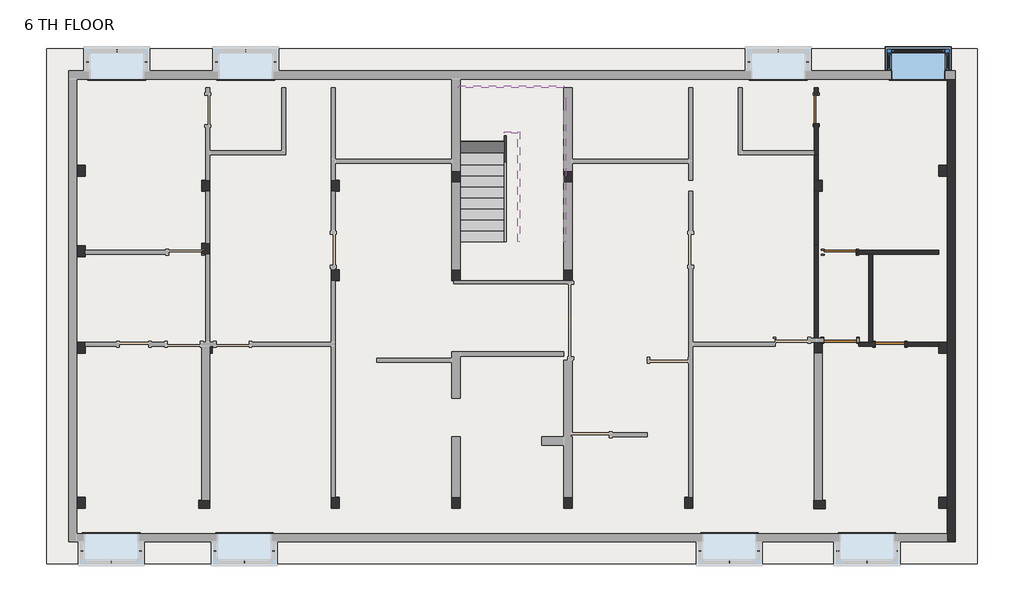
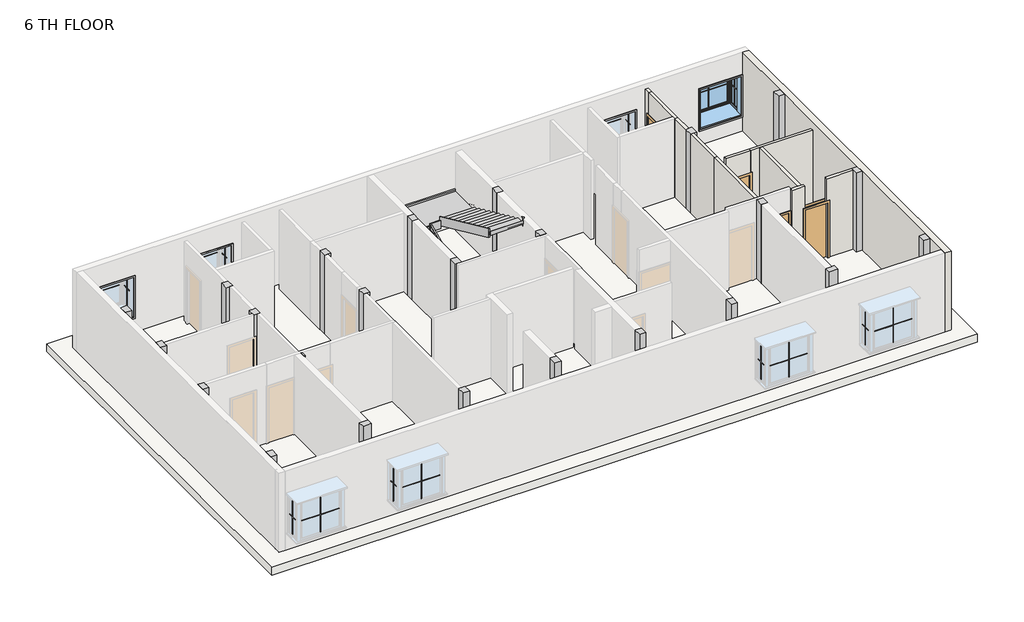
# One storey, part 2 of 2: 32 proxies, 24 columns, 11 walls, 6 members, 4 doors, 1 slab, 1 stair flight, 1 window.
"""IFC4 building model written with IfcOpenShell, lengths in millimetres."""

from ifc_helpers import new_model, si_unit, frame, origin, place, context, project, spatial, polyline, outline, extrude, faceted_brep, transform, mapped, element, save
from components import m_muntin_pattern_2x2_m_muntin_pattern_2x2_c1fd4460, m_muntin_pattern_2x2_m_muntin_pattern_2x2_777b163a, m_trim_window_interior_flat_picture_frame_44e8afef, column_1c121444, door_1991e9a2, door_a431d384, door_82def9da, m_door_single_panel_3_x7_f8176753, stair_flight_f18b4829, window_19bbd869

model = new_model("IFC4")

# Units and contexts
model_context = context("Model", 3, world=origin())
ifc_project = project(units=[si_unit("LENGTHUNIT", "METRE", prefix="MILLI")], contexts=[model_context])

# Site, building, storey
site = spatial("IfcSite", under=ifc_project)
building = spatial("IfcBuilding", under=site)
storey = spatial("IfcBuildingStorey", under=building, Name="6 TH FLOOR", Elevation=22402.8)

# Proxies
placement = place(None, origin())
m_muntin_pattern_2x2_m_muntin_pattern_2x2_shape = m_muntin_pattern_2x2_m_muntin_pattern_2x2_c1fd4460(model_context)
element("IfcBuildingElementProxy", 1, Name="M_Muntin Pattern_2x2 : M_Muntin Pattern_2x2", ObjectType="M_Muntin Pattern_2x2 : M_Muntin Pattern_2x2", at=placement, inside=storey, context=model_context, shape_type="MappedRepresentation", body=[
    mapped(m_muntin_pattern_2x2_m_muntin_pattern_2x2_shape, transform((-11500.7987957, -5499.9182661, 23123.45), x_axis=(-1.0, 0.0, 0.0), y_axis=(0.0, -1.0, 0.0), z_axis=(0.0, 0.0, 1.0))),
])
element("IfcBuildingElementProxy", 2, Name="M_Muntin Pattern_2x2 : M_Muntin Pattern_2x2", ObjectType="M_Muntin Pattern_2x2 : M_Muntin Pattern_2x2", at=placement, inside=storey, context=model_context, shape_type="MappedRepresentation", body=[
    mapped(m_muntin_pattern_2x2_m_muntin_pattern_2x2_shape, transform((-7819.250543, -5499.9182661, 23123.45), x_axis=(-1.0, 0.0, 0.0), y_axis=(0.0, -1.0, 0.0), z_axis=(0.0, 0.0, 1.0))),
])
element("IfcBuildingElementProxy", 3, Name="M_Muntin Pattern_2x2 : M_Muntin Pattern_2x2", ObjectType="M_Muntin Pattern_2x2 : M_Muntin Pattern_2x2", at=placement, inside=storey, context=model_context, shape_type="MappedRepresentation", body=[
    mapped(m_muntin_pattern_2x2_m_muntin_pattern_2x2_shape, transform((5599.7512082, -5499.9182661, 23123.45), x_axis=(-1.0, 0.0, 0.0), y_axis=(0.0, -1.0, 0.0), z_axis=(0.0, 0.0, 1.0))),
])
element("IfcBuildingElementProxy", 4, Name="M_Muntin Pattern_2x2 : M_Muntin Pattern_2x2", ObjectType="M_Muntin Pattern_2x2 : M_Muntin Pattern_2x2", at=placement, inside=storey, context=model_context, shape_type="MappedRepresentation", body=[
    mapped(m_muntin_pattern_2x2_m_muntin_pattern_2x2_shape, transform((9408.6146942, -5499.9182662, 23123.45), x_axis=(-1.0, 0.0, 0.0), y_axis=(0.0, -1.0, 0.0), z_axis=(0.0, 0.0, 1.0))),
])
element("IfcBuildingElementProxy", 5, Name="M_Muntin Pattern_2x2 : M_Muntin Pattern_2x2", ObjectType="M_Muntin Pattern_2x2 : M_Muntin Pattern_2x2", at=placement, inside=storey, context=model_context, shape_type="MappedRepresentation", body=[
    mapped(m_muntin_pattern_2x2_m_muntin_pattern_2x2_shape, transform((-11348.3987957, 8647.7317329, 23123.45), x_axis=(1.0, 0.0, 0.0), y_axis=(0.0, 1.0, 0.0), z_axis=(0.0, 0.0, 1.0))),
])
element("IfcBuildingElementProxy", 6, Name="M_Muntin Pattern_2x2 : M_Muntin Pattern_2x2", ObjectType="M_Muntin Pattern_2x2 : M_Muntin Pattern_2x2", at=placement, inside=storey, context=model_context, shape_type="MappedRepresentation", body=[
    mapped(m_muntin_pattern_2x2_m_muntin_pattern_2x2_shape, transform((-7779.6987993, 8647.7317329, 23123.45), x_axis=(1.0, 0.0, 0.0), y_axis=(0.0, 1.0, 0.0), z_axis=(0.0, 0.0, 1.0))),
])
element("IfcBuildingElementProxy", 7, Name="M_Muntin Pattern_2x2 : M_Muntin Pattern_2x2", ObjectType="M_Muntin Pattern_2x2 : M_Muntin Pattern_2x2", at=placement, inside=storey, context=model_context, shape_type="MappedRepresentation", body=[
    mapped(m_muntin_pattern_2x2_m_muntin_pattern_2x2_shape, transform((6952.301208, 8647.7317329, 23123.45), x_axis=(1.0, 0.0, 0.0), y_axis=(0.0, 1.0, 0.0), z_axis=(0.0, 0.0, 1.0))),
])
element("IfcBuildingElementProxy", 8, Name="M_Muntin Pattern_2x2 : M_Muntin Pattern_2x2", ObjectType="M_Muntin Pattern_2x2 : M_Muntin Pattern_2x2", at=placement, inside=storey, context=model_context, shape_type="MappedRepresentation", body=[
    mapped(m_muntin_pattern_2x2_m_muntin_pattern_2x2_shape, transform((10825.8012075, 8647.7317329, 23123.45), x_axis=(1.0, 0.0, 0.0), y_axis=(0.0, 1.0, 0.0), z_axis=(0.0, 0.0, 1.0))),
])
m_muntin_pattern_2x2_m_muntin_pattern_2x2_2_shape = m_muntin_pattern_2x2_m_muntin_pattern_2x2_777b163a(model_context)
element("IfcBuildingElementProxy", 9, Name="M_Muntin Pattern_2x2 : M_Muntin Pattern_2x2", ObjectType="M_Muntin Pattern_2x2 : M_Muntin Pattern_2x2", at=placement, inside=storey, context=model_context, shape_type="MappedRepresentation", body=[
    mapped(m_muntin_pattern_2x2_m_muntin_pattern_2x2_2_shape, transform((-10690.4737957, -5190.3932661, 23123.45), x_axis=(0.0, 1.0, 0.0), y_axis=(-1.0, 0.0, 0.0), z_axis=(0.0, 0.0, 1.0))),
])
element("IfcBuildingElementProxy", 10, Name="M_Muntin Pattern_2x2 : M_Muntin Pattern_2x2", ObjectType="M_Muntin Pattern_2x2 : M_Muntin Pattern_2x2", at=placement, inside=storey, context=model_context, shape_type="MappedRepresentation", body=[
    mapped(m_muntin_pattern_2x2_m_muntin_pattern_2x2_2_shape, transform((-12311.1237957, -5190.3932661, 23123.45), x_axis=(0.0, -1.0, 0.0), y_axis=(1.0, 0.0, 0.0), z_axis=(0.0, 0.0, 1.0))),
])
element("IfcBuildingElementProxy", 11, Name="M_Muntin Pattern_2x2 : M_Muntin Pattern_2x2", ObjectType="M_Muntin Pattern_2x2 : M_Muntin Pattern_2x2", at=placement, inside=storey, context=model_context, shape_type="MappedRepresentation", body=[
    mapped(m_muntin_pattern_2x2_m_muntin_pattern_2x2_2_shape, transform((-7008.925543, -5190.3932661, 23123.45), x_axis=(0.0, 1.0, 0.0), y_axis=(-1.0, 0.0, 0.0), z_axis=(0.0, 0.0, 1.0))),
])
element("IfcBuildingElementProxy", 12, Name="M_Muntin Pattern_2x2 : M_Muntin Pattern_2x2", ObjectType="M_Muntin Pattern_2x2 : M_Muntin Pattern_2x2", at=placement, inside=storey, context=model_context, shape_type="MappedRepresentation", body=[
    mapped(m_muntin_pattern_2x2_m_muntin_pattern_2x2_2_shape, transform((-8629.575543, -5190.3932661, 23123.45), x_axis=(0.0, -1.0, 0.0), y_axis=(1.0, 0.0, 0.0), z_axis=(0.0, 0.0, 1.0))),
])
element("IfcBuildingElementProxy", 13, Name="M_Muntin Pattern_2x2 : M_Muntin Pattern_2x2", ObjectType="M_Muntin Pattern_2x2 : M_Muntin Pattern_2x2", at=placement, inside=storey, context=model_context, shape_type="MappedRepresentation", body=[
    mapped(m_muntin_pattern_2x2_m_muntin_pattern_2x2_2_shape, transform((6410.0762082, -5190.3932661, 23123.45), x_axis=(0.0, 1.0, 0.0), y_axis=(-1.0, 0.0, 0.0), z_axis=(0.0, 0.0, 1.0))),
])
element("IfcBuildingElementProxy", 14, Name="M_Muntin Pattern_2x2 : M_Muntin Pattern_2x2", ObjectType="M_Muntin Pattern_2x2 : M_Muntin Pattern_2x2", at=placement, inside=storey, context=model_context, shape_type="MappedRepresentation", body=[
    mapped(m_muntin_pattern_2x2_m_muntin_pattern_2x2_2_shape, transform((4789.4262082, -5190.3932661, 23123.45), x_axis=(0.0, -1.0, 0.0), y_axis=(1.0, 0.0, 0.0), z_axis=(0.0, 0.0, 1.0))),
])
element("IfcBuildingElementProxy", 15, Name="M_Muntin Pattern_2x2 : M_Muntin Pattern_2x2", ObjectType="M_Muntin Pattern_2x2 : M_Muntin Pattern_2x2", at=placement, inside=storey, context=model_context, shape_type="MappedRepresentation", body=[
    mapped(m_muntin_pattern_2x2_m_muntin_pattern_2x2_2_shape, transform((10218.9396942, -5190.3932662, 23123.45), x_axis=(0.0, 1.0, 0.0), y_axis=(-1.0, 0.0, 0.0), z_axis=(0.0, 0.0, 1.0))),
])
element("IfcBuildingElementProxy", 16, Name="M_Muntin Pattern_2x2 : M_Muntin Pattern_2x2", ObjectType="M_Muntin Pattern_2x2 : M_Muntin Pattern_2x2", at=placement, inside=storey, context=model_context, shape_type="MappedRepresentation", body=[
    mapped(m_muntin_pattern_2x2_m_muntin_pattern_2x2_2_shape, transform((8598.2896942, -5190.3932661, 23123.45), x_axis=(0.0, -1.0, 0.0), y_axis=(1.0, 0.0, 0.0), z_axis=(0.0, 0.0, 1.0))),
])
element("IfcBuildingElementProxy", 17, Name="M_Muntin Pattern_2x2 : M_Muntin Pattern_2x2", ObjectType="M_Muntin Pattern_2x2 : M_Muntin Pattern_2x2", at=placement, inside=storey, context=model_context, shape_type="MappedRepresentation", body=[
    mapped(m_muntin_pattern_2x2_m_muntin_pattern_2x2_2_shape, transform((-12158.7237957, 8338.2067329, 23123.45), x_axis=(0.0, -1.0, 0.0), y_axis=(1.0, 0.0, 0.0), z_axis=(0.0, 0.0, 1.0))),
])
element("IfcBuildingElementProxy", 18, Name="M_Muntin Pattern_2x2 : M_Muntin Pattern_2x2", ObjectType="M_Muntin Pattern_2x2 : M_Muntin Pattern_2x2", at=placement, inside=storey, context=model_context, shape_type="MappedRepresentation", body=[
    mapped(m_muntin_pattern_2x2_m_muntin_pattern_2x2_2_shape, transform((-10538.0737957, 8338.2067329, 23123.45), x_axis=(0.0, 1.0, 0.0), y_axis=(-1.0, 0.0, 0.0), z_axis=(0.0, 0.0, 1.0))),
])
element("IfcBuildingElementProxy", 19, Name="M_Muntin Pattern_2x2 : M_Muntin Pattern_2x2", ObjectType="M_Muntin Pattern_2x2 : M_Muntin Pattern_2x2", at=placement, inside=storey, context=model_context, shape_type="MappedRepresentation", body=[
    mapped(m_muntin_pattern_2x2_m_muntin_pattern_2x2_2_shape, transform((-8590.0237993, 8338.2067329, 23123.45), x_axis=(0.0, -1.0, 0.0), y_axis=(1.0, 0.0, 0.0), z_axis=(0.0, 0.0, 1.0))),
])
element("IfcBuildingElementProxy", 20, Name="M_Muntin Pattern_2x2 : M_Muntin Pattern_2x2", ObjectType="M_Muntin Pattern_2x2 : M_Muntin Pattern_2x2", at=placement, inside=storey, context=model_context, shape_type="MappedRepresentation", body=[
    mapped(m_muntin_pattern_2x2_m_muntin_pattern_2x2_2_shape, transform((-6969.3737993, 8338.2067329, 23123.45), x_axis=(0.0, 1.0, 0.0), y_axis=(-1.0, 0.0, 0.0), z_axis=(0.0, 0.0, 1.0))),
])
element("IfcBuildingElementProxy", 21, Name="M_Muntin Pattern_2x2 : M_Muntin Pattern_2x2", ObjectType="M_Muntin Pattern_2x2 : M_Muntin Pattern_2x2", at=placement, inside=storey, context=model_context, shape_type="MappedRepresentation", body=[
    mapped(m_muntin_pattern_2x2_m_muntin_pattern_2x2_2_shape, transform((6141.976208, 8338.2067329, 23123.45), x_axis=(0.0, -1.0, 0.0), y_axis=(1.0, 0.0, 0.0), z_axis=(0.0, 0.0, 1.0))),
])
element("IfcBuildingElementProxy", 22, Name="M_Muntin Pattern_2x2 : M_Muntin Pattern_2x2", ObjectType="M_Muntin Pattern_2x2 : M_Muntin Pattern_2x2", at=placement, inside=storey, context=model_context, shape_type="MappedRepresentation", body=[
    mapped(m_muntin_pattern_2x2_m_muntin_pattern_2x2_2_shape, transform((7762.626208, 8338.2067329, 23123.45), x_axis=(0.0, 1.0, 0.0), y_axis=(-1.0, 0.0, 0.0), z_axis=(0.0, 0.0, 1.0))),
])
element("IfcBuildingElementProxy", 23, Name="M_Muntin Pattern_2x2 : M_Muntin Pattern_2x2", ObjectType="M_Muntin Pattern_2x2 : M_Muntin Pattern_2x2", at=placement, inside=storey, context=model_context, shape_type="MappedRepresentation", body=[
    mapped(m_muntin_pattern_2x2_m_muntin_pattern_2x2_2_shape, transform((10015.4762075, 8338.2067329, 23123.45), x_axis=(0.0, -1.0, 0.0), y_axis=(1.0, 0.0, 0.0), z_axis=(0.0, 0.0, 1.0))),
])
element("IfcBuildingElementProxy", 24, Name="M_Muntin Pattern_2x2 : M_Muntin Pattern_2x2", ObjectType="M_Muntin Pattern_2x2 : M_Muntin Pattern_2x2", at=placement, inside=storey, context=model_context, shape_type="MappedRepresentation", body=[
    mapped(m_muntin_pattern_2x2_m_muntin_pattern_2x2_2_shape, transform((11636.1262075, 8338.2067329, 23123.45), x_axis=(0.0, 1.0, 0.0), y_axis=(-1.0, 0.0, 0.0), z_axis=(0.0, 0.0, 1.0))),
])
m_trim_window_interior_flat_picture_frame_shape = m_trim_window_interior_flat_picture_frame_44e8afef(model_context)
element("IfcBuildingElementProxy", 25, Name="M_Trim-Window-Interior-Flat : Picture Frame", ObjectType="M_Trim-Window-Interior-Flat : Picture Frame", at=placement, inside=storey, context=model_context, shape_type="MappedRepresentation", body=[
    mapped(m_trim_window_interior_flat_picture_frame_shape, transform((-11500.7987957, -4712.5932661, 24553.6), x_axis=(-1.0, 0.0, 0.0), y_axis=(0.0, 0.0, 1.0), z_axis=(0.0, 1.0, 0.0))),
])
element("IfcBuildingElementProxy", 26, Name="M_Trim-Window-Interior-Flat : Picture Frame", ObjectType="M_Trim-Window-Interior-Flat : Picture Frame", at=placement, inside=storey, context=model_context, shape_type="MappedRepresentation", body=[
    mapped(m_trim_window_interior_flat_picture_frame_shape, transform((-7819.250543, -4712.5932661, 24553.6), x_axis=(-1.0, 0.0, 0.0), y_axis=(0.0, 0.0, 1.0), z_axis=(0.0, 1.0, 0.0))),
])
element("IfcBuildingElementProxy", 27, Name="M_Trim-Window-Interior-Flat : Picture Frame", ObjectType="M_Trim-Window-Interior-Flat : Picture Frame", at=placement, inside=storey, context=model_context, shape_type="MappedRepresentation", body=[
    mapped(m_trim_window_interior_flat_picture_frame_shape, transform((5599.7512082, -4712.5932661, 24553.6), x_axis=(-1.0, 0.0, 0.0), y_axis=(0.0, 0.0, 1.0), z_axis=(0.0, 1.0, 0.0))),
])
element("IfcBuildingElementProxy", 28, Name="M_Trim-Window-Interior-Flat : Picture Frame", ObjectType="M_Trim-Window-Interior-Flat : Picture Frame", at=placement, inside=storey, context=model_context, shape_type="MappedRepresentation", body=[
    mapped(m_trim_window_interior_flat_picture_frame_shape, transform((9408.6146942, -4712.5932661, 24553.6), x_axis=(-1.0, 0.0, 0.0), y_axis=(0.0, 0.0, 1.0), z_axis=(0.0, 1.0, 0.0))),
])
element("IfcBuildingElementProxy", 29, Name="M_Trim-Window-Interior-Flat : Picture Frame", ObjectType="M_Trim-Window-Interior-Flat : Picture Frame", at=placement, inside=storey, context=model_context, shape_type="MappedRepresentation", body=[
    mapped(m_trim_window_interior_flat_picture_frame_shape, transform((-11348.3987957, 7860.4067329, 24553.6), x_axis=(1.0, 0.0, 0.0), y_axis=(0.0, 0.0, 1.0), z_axis=(0.0, -1.0, 0.0))),
])
element("IfcBuildingElementProxy", 30, Name="M_Trim-Window-Interior-Flat : Picture Frame", ObjectType="M_Trim-Window-Interior-Flat : Picture Frame", at=placement, inside=storey, context=model_context, shape_type="MappedRepresentation", body=[
    mapped(m_trim_window_interior_flat_picture_frame_shape, transform((-7779.6987993, 7860.4067329, 24553.6), x_axis=(1.0, 0.0, 0.0), y_axis=(0.0, 0.0, 1.0), z_axis=(0.0, -1.0, 0.0))),
])
element("IfcBuildingElementProxy", 31, Name="M_Trim-Window-Interior-Flat : Picture Frame", ObjectType="M_Trim-Window-Interior-Flat : Picture Frame", at=placement, inside=storey, context=model_context, shape_type="MappedRepresentation", body=[
    mapped(m_trim_window_interior_flat_picture_frame_shape, transform((6952.301208, 7860.4067329, 24553.6), x_axis=(1.0, 0.0, 0.0), y_axis=(0.0, 0.0, 1.0), z_axis=(0.0, -1.0, 0.0))),
])
element("IfcBuildingElementProxy", 32, Name="M_Trim-Window-Interior-Flat : Picture Frame", ObjectType="M_Trim-Window-Interior-Flat : Picture Frame", at=placement, inside=storey, context=model_context, shape_type="MappedRepresentation", body=[
    mapped(m_trim_window_interior_flat_picture_frame_shape, transform((10825.8012075, 7860.4067329, 24553.6), x_axis=(1.0, 0.0, 0.0), y_axis=(0.0, 0.0, 1.0), z_axis=(0.0, -1.0, 0.0))),
])

# Columns
element("IfcColumn", 33, ObjectType="Rectangular Column : 1'X 9\"", at=placement, inside=storey, context=model_context, shape_type="SweptSolid", body=[
    extrude(outline(polyline([(-12224.6987957, -3709.2932671), (-12224.6987957, -4014.0932671), (-12453.2987957, -4014.0932671), (-12453.2987957, -3709.2932671), (-12224.6987957, -3709.2932671)])), frame((0.0, 0.0, 22402.8), z_axis=(0.0, 0.0, 1.0), x_axis=(1.0, 0.0, 0.0)), (0.0, 0.0, 1.0), 3048.0),
])
element("IfcColumn", 34, ObjectType="Rectangular Column : 1'X 9\"", at=placement, inside=storey, context=model_context, shape_type="SweptSolid", body=[
    extrude(outline(polyline([(-12224.6987957, 583.3067334), (-12224.6987957, 278.5067334), (-12453.2987957, 278.5067334), (-12453.2987957, 583.3067334), (-12224.6987957, 583.3067334)])), frame((0.0, 0.0, 22402.8), z_axis=(0.0, 0.0, 1.0), x_axis=(1.0, 0.0, 0.0)), (0.0, 0.0, 1.0), 3048.0),
])
element("IfcColumn", 35, ObjectType="Rectangular Column : 1'X 9\"", at=placement, inside=storey, context=model_context, shape_type="SweptSolid", body=[
    extrude(outline(polyline([(-12224.6987957, 3256.6567332), (-12224.6987957, 2951.8567332), (-12453.2987957, 2951.8567332), (-12453.2987957, 3256.6567332), (-12224.6987957, 3256.6567332)])), frame((0.0, 0.0, 22402.8), z_axis=(0.0, 0.0, 1.0), x_axis=(1.0, 0.0, 0.0)), (0.0, 0.0, 1.0), 3048.0),
])
element("IfcColumn", 36, ObjectType="Rectangular Column : 1'X 9\"", at=placement, inside=storey, context=model_context, shape_type="Brep", body=[
    faceted_brep([(-8770.2987992, 5066.406733, 22402.8), (-8770.2987992, 4761.606733, 22402.8), (-8884.5987992, 4761.606733, 22402.8), (-8998.8987992, 4761.606733, 22402.8), (-8998.8987992, 5066.406733, 22402.8), (-8884.5987992, 5066.406733, 22402.8), (-8770.2987992, 5066.406733, 25450.8), (-8770.2987992, 4761.606733, 25450.8), (-8884.5987992, 4761.606733, 25450.8), (-8998.8987992, 4761.606733, 25450.8), (-8998.8987992, 5066.406733, 25450.8), (-8884.5987992, 5066.406733, 25450.8)], [[[0, 1, 2, 3, 4, 5]], [[6, 7, 1, 0]], [[7, 8, 9, 3, 2, 1]], [[9, 10, 4, 3]], [[10, 11, 6, 0, 5, 4]], [[6, 11, 10, 9, 8, 7]]]),
])
element("IfcColumn", 37, ObjectType="Rectangular Column : 1'X 9\"", at=placement, inside=storey, context=model_context, shape_type="Brep", body=[
    faceted_brep([(-8770.2987992, 3326.5067332, 22402.8), (-8770.2987992, 3021.7067332, 22402.8), (-8884.598796, 3021.7067332, 22402.8), (-8998.8987992, 3021.7067332, 22402.8), (-8998.8987992, 3326.5067332, 22402.8), (-8884.5987992, 3326.5067332, 22402.8), (-8770.2987992, 3326.5067332, 25450.8), (-8770.2987992, 3021.7067332, 25450.8), (-8884.598796, 3021.7067332, 25450.8), (-8998.8987992, 3021.7067332, 25450.8), (-8998.8987992, 3326.5067332, 25450.8), (-8884.5987992, 3326.5067332, 25450.8)], [[[0, 1, 2, 3, 4, 5]], [[6, 7, 1, 0]], [[7, 8, 9, 3, 2, 1]], [[9, 10, 4, 3]], [[10, 11, 6, 0, 5, 4]], [[6, 11, 10, 9, 8, 7]]]),
])
element("IfcColumn", 38, ObjectType="Rectangular Column : 1'X 9\"", at=placement, inside=storey, context=model_context, shape_type="SweptSolid", body=[
    extrude(outline(polyline([(-8713.148796, 278.5067334), (-8771.750543, 278.5067334), (-8771.750543, 469.0067334), (-8713.148796, 469.0067334), (-8713.148796, 278.5067334)])), frame((0.0, 0.0, 22402.8), z_axis=(0.0, 0.0, 1.0), x_axis=(1.0, 0.0, 0.0)), (0.0, 0.0, 1.0), 3048.0),
])
element("IfcColumn", 39, ObjectType="Rectangular Column : 1'X 9\"", at=placement, inside=storey, context=model_context, shape_type="Brep", body=[
    faceted_brep([(-5188.8987995, 5066.406733, 22402.8), (-5188.8987995, 4761.606733, 22402.8), (-5303.1987995, 4761.606733, 22402.8), (-5417.4987995, 4761.606733, 22402.8), (-5417.4987995, 5066.406733, 22402.8), (-5303.1987995, 5066.406733, 22402.8), (-5188.8987995, 5066.406733, 25450.8), (-5188.8987995, 4761.606733, 25450.8), (-5303.1987995, 4761.606733, 25450.8), (-5417.4987995, 4761.606733, 25450.8), (-5417.4987995, 5066.406733, 25450.8), (-5303.1987995, 5066.406733, 25450.8)], [[[0, 1, 2, 3, 4, 5]], [[6, 7, 1, 0]], [[7, 8, 9, 3, 2, 1]], [[9, 10, 4, 3]], [[10, 11, 6, 0, 5, 4]], [[6, 11, 10, 9, 8, 7]]]),
])
element("IfcColumn", 40, ObjectType="Rectangular Column : 1'X 9\"", at=placement, inside=storey, context=model_context, shape_type="Brep", body=[
    faceted_brep([(-5188.8987995, 2589.9067802, 22402.8), (-5188.8987995, 2285.1067802, 22402.8), (-5303.1987995, 2285.1067802, 22402.8), (-5417.4987995, 2285.1067802, 22402.8), (-5417.4987995, 2589.9067802, 22402.8), (-5303.1987995, 2589.9067802, 22402.8), (-5188.8987995, 2589.9067802, 25450.8), (-5188.8987995, 2285.1067802, 25450.8), (-5303.1987995, 2285.1067802, 25450.8), (-5417.4987995, 2285.1067802, 25450.8), (-5417.4987995, 2589.9067802, 25450.8), (-5303.1987995, 2589.9067802, 25450.8)], [[[0, 1, 2, 3, 4, 5]], [[6, 7, 1, 0]], [[7, 8, 9, 3, 2, 1]], [[9, 10, 4, 3]], [[10, 11, 6, 0, 5, 4]], [[6, 11, 10, 9, 8, 7]]]),
])
element("IfcColumn", 41, ObjectType="Rectangular Column : 1'X 9\"", at=placement, inside=storey, context=model_context, shape_type="Brep", body=[
    faceted_brep([(-5188.8987963, -3709.2932193, 22402.8), (-5188.8987963, -4014.0932193, 22402.8), (-5417.4987963, -4014.0932193, 22402.8), (-5417.4987963, -3709.2932193, 22402.8), (-5303.1987995, -3709.2932193, 22402.8), (-5188.8987963, -3709.2932193, 25450.8), (-5188.8987963, -4014.0932193, 25450.8), (-5417.4987963, -4014.0932193, 25450.8), (-5417.4987963, -3709.2932193, 25450.8), (-5303.1987995, -3709.2932193, 25450.8)], [[[0, 1, 2, 3, 4]], [[5, 6, 1, 0]], [[6, 7, 2, 1]], [[7, 8, 3, 2]], [[8, 9, 5, 0, 4, 3]], [[5, 9, 8, 7, 6]]]),
])
element("IfcColumn", 42, ObjectType="Rectangular Column : 1'X 9\"", at=placement, inside=storey, context=model_context, shape_type="SweptSolid", body=[
    extrude(outline(polyline([(1250.0012085, -3709.2932193), (1250.0012085, -4014.0932193), (1021.4012085, -4014.0932193), (1021.4012085, -3709.2932193), (1250.0012085, -3709.2932193)])), frame((0.0, 0.0, 22402.8), z_axis=(0.0, 0.0, 1.0), x_axis=(1.0, 0.0, 0.0)), (0.0, 0.0, 1.0), 3048.0),
])
element("IfcColumn", 43, ObjectType="Rectangular Column : 1'X 9\"", at=placement, inside=storey, context=model_context, shape_type="Brep", body=[
    faceted_brep([(4590.1012082, -3709.2932193, 22402.8), (4590.1012082, -4014.0932193, 22402.8), (4361.5012082, -4014.0932193, 22402.8), (4361.5012082, -3709.2932193, 22402.8), (4475.8012082, -3709.2932193, 22402.8), (4590.1012082, -3709.2932193, 25450.8), (4590.1012082, -4014.0932193, 25450.8), (4361.5012082, -4014.0932193, 25450.8), (4361.5012082, -3709.2932193, 25450.8), (4475.8012082, -3709.2932193, 25450.8)], [[[0, 1, 2, 3, 4]], [[5, 6, 1, 0]], [[6, 7, 2, 1]], [[7, 8, 3, 2]], [[8, 9, 5, 0, 4, 3]], [[5, 9, 8, 7, 6]]]),
])
element("IfcColumn", 44, ObjectType="Rectangular Column : 1'X 9\"", at=placement, inside=storey, context=model_context, shape_type="SweptSolid", body=[
    extrude(outline(polyline([(11625.9012075, -3709.2932671), (11625.9012075, -4014.0932671), (11397.3012075, -4014.0932671), (11397.3012075, -3709.2932671), (11625.9012075, -3709.2932671)])), frame((0.0, 0.0, 22402.8), z_axis=(0.0, 0.0, 1.0), x_axis=(1.0, 0.0, 0.0)), (0.0, 0.0, 1.0), 3048.0),
])
element("IfcColumn", 45, ObjectType="Rectangular Column : 1'X 9\"", at=placement, inside=storey, context=model_context, shape_type="Brep", body=[
    faceted_brep([(11625.9012075, 583.3067295, 22402.8), (11625.9012075, 278.5067295, 22402.8), (11397.3012075, 278.5067295, 22402.8), (11397.3012075, 469.0067295, 22402.8), (11397.3012075, 583.3067295, 22402.8), (11625.9012075, 583.3067295, 25450.8), (11625.9012075, 278.5067295, 25450.8), (11397.3012075, 278.5067295, 25450.8), (11397.3012075, 469.0067295, 25450.8), (11397.3012075, 583.3067295, 25450.8)], [[[0, 1, 2, 3, 4]], [[5, 6, 1, 0]], [[6, 7, 2, 1]], [[7, 8, 9, 4, 3, 2]], [[9, 5, 0, 4]], [[5, 9, 8, 7, 6]]]),
])
element("IfcColumn", 46, ObjectType="Rectangular Column : 1'X 9\"", at=placement, inside=storey, context=model_context, shape_type="SweptSolid", body=[
    extrude(outline(polyline([(11625.9012075, 5479.1567329), (11625.9012075, 5174.3567329), (11397.3012075, 5174.3567329), (11397.3012075, 5479.1567329), (11625.9012075, 5479.1567329)])), frame((0.0, 0.0, 22402.8), z_axis=(0.0, 0.0, 1.0), x_axis=(1.0, 0.0, 0.0)), (0.0, 0.0, 1.0), 3048.0),
])
element("IfcColumn", 47, ObjectType="Rectangular Column : 1'X 9\"", at=placement, inside=storey, context=model_context, shape_type="Brep", body=[
    faceted_brep([(8172.5040565, 5065.4824989, 22402.8), (8172.5040565, 4760.6824989, 22402.8), (8057.2012047, 4760.6824989, 22402.8), (7943.9040565, 4760.6824989, 22402.8), (7943.9040565, 5065.4824989, 22402.8), (8058.2040565, 5065.4824989, 22402.8), (8172.5040565, 5065.4824989, 25450.8), (8172.5040565, 4760.6824989, 25450.8), (8057.2012047, 4760.6824989, 25450.8), (7943.9040565, 4760.6824989, 25450.8), (7943.9040565, 5065.4824989, 25450.8), (8058.2040565, 5065.4824989, 25450.8)], [[[0, 1, 2, 3, 4, 5]], [[6, 7, 1, 0]], [[7, 8, 9, 3, 2, 1]], [[9, 10, 4, 3]], [[10, 11, 6, 0, 5, 4]], [[6, 11, 10, 9, 8, 7]]]),
])
element("IfcColumn", 48, ObjectType="Rectangular Column : 1'X 9\"", at=placement, inside=storey, context=model_context, shape_type="Brep", body=[
    faceted_brep([(8171.5012047, 583.3067334, 22402.8), (8171.5012047, 278.5067334, 22402.8), (7942.9012047, 278.5067334, 22402.8), (7942.9012047, 583.3067334, 22402.8), (8000.0512079, 583.3067334, 22402.8), (8171.5012047, 583.3067334, 25450.8), (8171.5012047, 278.5067334, 25450.8), (7942.9012047, 278.5067334, 25450.8), (7942.9012047, 583.3067334, 25450.8), (8000.0512079, 583.3067334, 25450.8)], [[[0, 1, 2, 3, 4]], [[5, 6, 1, 0]], [[6, 7, 2, 1]], [[7, 8, 3, 2]], [[8, 9, 5, 0, 4, 3]], [[5, 9, 8, 7, 6]]]),
])
element("IfcColumn", 49, ObjectType="Rectangular Column : 1'X 9\"", at=placement, inside=storey, context=model_context, shape_type="Brep", body=[
    faceted_brep([(-9076.550543, -3785.4932196, 22402.8), (-9000.350543, -3785.4932196, 22402.8), (-8771.750543, -3785.4932196, 22402.8), (-8771.750543, -4014.0932196, 22402.8), (-9076.550543, -4014.0932196, 22402.8), (-9076.550543, -3785.4932196, 25450.8), (-9000.350543, -3785.4932196, 25450.8), (-8771.750543, -3785.4932196, 25450.8), (-8771.750543, -4014.0932196, 25450.8), (-9076.550543, -4014.0932196, 25450.8)], [[[0, 1, 2, 3, 4]], [[5, 6, 7, 2, 1, 0]], [[7, 8, 3, 2]], [[8, 9, 4, 3]], [[9, 5, 0, 4]], [[5, 9, 8, 7, 6]]]),
])
element("IfcColumn", 50, ObjectType="Rectangular Column : 1'X 9\"", at=placement, inside=storey, context=model_context, shape_type="SweptSolid", body=[
    extrude(outline(polyline([(-12453.2987957, 5174.3567339), (-12453.2987957, 5479.1567339), (-12224.6987957, 5479.1567339), (-12224.6987957, 5174.3567339), (-12453.2987957, 5174.3567339)])), frame((0.0, 0.0, 22402.8), z_axis=(0.0, 0.0, 1.0), x_axis=(1.0, 0.0, 0.0)), (0.0, 0.0, 1.0), 3048.0),
])
element("IfcColumn", 51, ObjectType="Rectangular Column : 1'X 9\"", at=placement, inside=storey, context=model_context, shape_type="SweptSolid", body=[
    extrude(outline(polyline([(-1845.5417538, 5320.4067329), (-1845.5417538, 5015.6067329), (-2074.1417538, 5015.6067329), (-2074.1417538, 5320.4067329), (-1845.5417538, 5320.4067329)])), frame((0.0, 0.0, 22402.8), z_axis=(0.0, 0.0, 1.0), x_axis=(1.0, 0.0, 0.0)), (0.0, 0.0, 1.0), 3048.0),
])
element("IfcColumn", 52, ObjectType="Rectangular Column : 1'X 9\"", at=placement, inside=storey, context=model_context, shape_type="SweptSolid", body=[
    extrude(outline(polyline([(1250.0012085, 5320.4067329), (1250.0012085, 5015.6067329), (1021.4012085, 5015.6067329), (1021.4012085, 5320.4067329), (1250.0012085, 5320.4067329)])), frame((0.0, 0.0, 22402.8), z_axis=(0.0, 0.0, 1.0), x_axis=(1.0, 0.0, 0.0)), (0.0, 0.0, 1.0), 3048.0),
])
element("IfcColumn", 53, ObjectType="Rectangular Column : 1'X 9\"", at=placement, inside=storey, context=model_context, shape_type="Brep", body=[
    faceted_brep([(-1845.5417538, 2589.906774, 22402.8), (-1845.5417538, 2285.106774, 22402.8), (-2020.2487998, 2285.106774, 22402.8), (-2074.1417538, 2285.106774, 22402.8), (-2074.1417538, 2589.906774, 22402.8), (-1845.5417538, 2589.906774, 25450.8), (-1845.5417538, 2285.106774, 25450.8), (-2020.2487998, 2285.106774, 25450.8), (-2074.1417538, 2285.106774, 25450.8), (-2074.1417538, 2589.906774, 25450.8)], [[[0, 1, 2, 3, 4]], [[5, 6, 1, 0]], [[6, 7, 8, 3, 2, 1]], [[8, 9, 4, 3]], [[9, 5, 0, 4]], [[5, 9, 8, 7, 6]]]),
])
element("IfcColumn", 54, ObjectType="Rectangular Column : 1'X 9\"", at=placement, inside=storey, context=model_context, shape_type="Brep", body=[
    faceted_brep([(1253.2582462, 2589.9067742, 22402.8), (1253.2582462, 2285.1067742, 22402.8), (1024.6582462, 2285.1067742, 22402.8), (1024.6582462, 2589.9067742, 22402.8), (1250.0012085, 2589.9067742, 22402.8), (1253.2582462, 2589.9067742, 25450.8), (1253.2582462, 2285.1067742, 25450.8), (1024.6582462, 2285.1067742, 25450.8), (1024.6582462, 2589.9067742, 25450.8), (1250.0012085, 2589.9067742, 25450.8)], [[[0, 1, 2, 3, 4]], [[5, 6, 1, 0]], [[6, 7, 2, 1]], [[7, 8, 3, 2]], [[8, 9, 5, 0, 4, 3]], [[5, 9, 8, 7, 6]]]),
])
element("IfcColumn", 55, ObjectType="Rectangular Column : 1'X 9\"", at=placement, inside=storey, context=model_context, shape_type="SweptSolid", body=[
    extrude(outline(polyline([(-1848.7987998, -3709.2932663), (-1848.7987998, -4014.0932663), (-2077.3987998, -4014.0932663), (-2077.3987998, -3709.2932663), (-1848.7987998, -3709.2932663)])), frame((0.0, 0.0, 22402.8), z_axis=(0.0, 0.0, 1.0), x_axis=(1.0, 0.0, 0.0)), (0.0, 0.0, 1.0), 3048.0),
])
column_shape = column_1c121444(model_context)
element("IfcColumn", 56, ObjectType="Rectangular Column : 1'X 9\"", at=placement, inside=storey, context=model_context, shape_type="MappedRepresentation", body=[
    mapped(column_shape, transform((8094.1646942, -3901.6914801, 0.0), x_axis=(0.0, 1.0, 0.0), y_axis=(-1.0, 0.0, 0.0), z_axis=(0.0, 0.0, 1.0))),
])

# Doors
door_shape = door_1991e9a2(model_context)
element("IfcDoor", 57, ObjectType="M_Door-Single-Panel : 2'11\"X7' 3", at=placement, inside=storey, context=model_context, shape_type="MappedRepresentation", body=[
    mapped(door_shape, transform((8664.274939, 3078.8567332, 22402.8), x_axis=(-1.0, 0.0, 0.0), y_axis=(0.0, -1.0, 0.0), z_axis=(0.0, 0.0, 1.0))),
])
door_2_shape = door_a431d384(model_context)
element("IfcDoor", 58, ObjectType="M_Door-Single-Panel : 2'7\"X7' 2", at=placement, inside=storey, context=model_context, shape_type="MappedRepresentation", body=[
    mapped(door_2_shape, transform((8000.0512079, 7021.3751452, 22402.8), x_axis=(0.0, 1.0, 0.0), y_axis=(-1.0, 0.0, 0.0), z_axis=(0.0, 0.0, 1.0))),
])
door_3_shape = door_82def9da(model_context)
element("IfcDoor", 59, ObjectType="M_Door-Single-Panel : 2'8\"X7'", at=placement, inside=storey, context=model_context, shape_type="MappedRepresentation", body=[
    mapped(door_3_shape, transform((10046.0486694, 526.1567295, 22402.8), x_axis=(-1.0, 0.0, 0.0), y_axis=(0.0, -1.0, 0.0), z_axis=(0.0, 0.0, 1.0))),
])
m_door_single_panel_3_x7_shape = m_door_single_panel_3_x7_f8176753(model_context)
element("IfcDoor", 60, ObjectType="M_Door-Single-Panel : 3'X7'", at=placement, inside=storey, context=model_context, shape_type="MappedRepresentation", body=[
    mapped(m_door_single_panel_3_x7_shape, transform((8666.8012079, 640.4567334, 22402.8), x_axis=(-1.0, 0.0, 0.0), y_axis=(0.0, -1.0, 0.0), z_axis=(0.0, 0.0, 1.0))),
])

# Members
element("IfcMember", 61, ObjectType="Stringer - 2\" Width", at=placement, inside=storey, context=model_context, shape_type="SweptSolid", body=[
    extrude(outline(polyline([(3364.6067329, 22402.8), (3364.6067329, 22602.6262721), (6445.4289342, 24003.0), (7182.0114168, 24003.0), (3661.5714168, 22402.8), (3364.6067329, 22402.8)])), frame((-1896.3417538, 0.0, 0.0), z_axis=(1.0, 0.0, 0.0), x_axis=(0.0, 1.0, 0.0)), (0.0, 0.0, 1.0), 50.8),
])
element("IfcMember", 62, ObjectType="Stringer - 2\" Width", at=placement, inside=storey, context=model_context, shape_type="SweptSolid", body=[
    extrude(outline(polyline([(-1896.3417538, 7631.8067329), (-1896.3417538, 7682.6067329), (1021.4012085, 7682.6067329), (1021.4012085, 7631.8067329), (-1896.3417538, 7631.8067329)])), frame((0.0, 0.0, 23698.2), z_axis=(0.0, 0.0, 1.0), x_axis=(1.0, 0.0, 0.0)), (0.0, 0.0, 1.0), 304.8),
])
element("IfcMember", 63, ObjectType="Stringer - 2\" Width", at=placement, inside=storey, context=model_context, shape_type="SweptSolid", body=[
    extrude(outline(polyline([(6618.562049, 23698.2), (3364.6067329, 25177.2705982), (3364.6067329, 25512.0808176), (7355.1445316, 23698.2), (6618.562049, 23698.2)])), frame((1021.4012085, 0.0, 0.0), z_axis=(1.0, 0.0, 0.0), x_axis=(0.0, 1.0, 0.0)), (0.0, 0.0, 1.0), 50.8),
])
element("IfcMember", 64, ObjectType="Stringer - 2\" Width", at=placement, inside=storey, context=model_context, shape_type="SweptSolid", body=[
    extrude(outline(polyline([(3364.6067329, 22402.8), (3364.6067329, 22602.6262721), (6361.8067329, 23964.9899085), (6361.8067329, 23630.1796892), (3661.5714168, 22402.8), (3364.6067329, 22402.8)])), frame((-629.5987998, 0.0, 0.0), z_axis=(1.0, 0.0, 0.0), x_axis=(0.0, 1.0, 0.0)), (0.0, 0.0, 1.0), 50.8),
])
element("IfcMember", 65, ObjectType="Stringer - 2\" Width", at=placement, inside=storey, context=model_context, shape_type="SweptSolid", body=[
    extrude(outline(polyline([(-629.5987998, 6361.8067329), (-629.5987998, 6412.6067329), (-248.5987915, 6412.6067329), (-248.5987915, 6361.8067329), (-629.5987998, 6361.8067329)])), frame((0.0, 0.0, 23698.2), z_axis=(0.0, 0.0, 1.0), x_axis=(1.0, 0.0, 0.0)), (0.0, 0.0, 1.0), 304.8),
])
element("IfcMember", 66, ObjectType="Stringer - 2\" Width", at=placement, inside=storey, context=model_context, shape_type="SweptSolid", body=[
    extrude(outline(polyline([(6412.6067329, 24126.6262721), (6412.6067329, 23791.8160528), (3364.6067329, 25177.2705982), (3364.6067329, 25512.0808176), (6412.6067329, 24126.6262721)])), frame((-248.5987915, 0.0, 0.0), z_axis=(1.0, 0.0, 0.0), x_axis=(0.0, 1.0, 0.0)), (0.0, 0.0, 1.0), 50.8),
])

# Slab
element("IfcSlab", 67, ObjectType="Generic - 12\"", at=placement, inside=storey, context=model_context, shape_type="SweptSolid", body=[
    extrude(outline(polyline([(12464.1012075, 8698.6067329), (12464.1012075, -5550.7932662), (-13291.4987957, -5550.7932662), (-13291.4987957, 8698.6067329), (12464.1012075, 8698.6067329)])), frame((0.0, 0.0, 22098.0), z_axis=(0.0, 0.0, 1.0), x_axis=(1.0, 0.0, 0.0)), (0.0, 0.0, 1.0), 304.8),
])

# Stair flight
stair_flight_shape = stair_flight_f18b4829(model_context)
element("IfcStairFlight", 68, ObjectType="2\" Tread 1\" Nosing 1/4\" Riser", at=placement, inside=storey, context=model_context, shape_type="MappedRepresentation", body=[
    mapped(stair_flight_shape, transform((0.0, 0.0, 0.0), x_axis=(1.0, 0.0, 0.0), y_axis=(0.0, 1.0, 0.0), z_axis=(0.0, 0.0, 1.0))),
])

# Walls
element("IfcWall", 69, ObjectType="4.5\"", at=placement, inside=storey, context=model_context, shape_type="SweptSolid", body=[
    extrude(outline(polyline([(22402.8, 9131.6486701), (25450.8, 9131.6486701), (25450.8, 8245.174939), (24536.4, 8245.174939), (24536.4, 9108.774939), (22402.8, 9108.774939), (22402.8, 9131.6486701)])), frame((0.0, 3021.7067332, 0.0), z_axis=(0.0, 1.0, 0.0), x_axis=(0.0, 0.0, 1.0)), (0.0, 0.0, 1.0), 114.3),
])
element("IfcWall", 70, ObjectType="4.5\"", at=placement, inside=storey, context=model_context, shape_type="Brep", body=[
    faceted_brep([(7942.9012079, 5764.9067329, 25450.8), (7942.9012079, 5879.2067329, 25450.8), (7942.9012079, 7415.0751452, 25450.8), (7942.9012079, 7415.0751452, 24536.4), (7942.9012079, 6627.6751452, 24536.4), (7942.9012079, 6627.6751452, 22402.8), (7942.9012079, 5879.2067329, 22402.8), (7942.9012079, 5764.9067329, 22402.8), (8057.2012079, 7415.0751452, 25450.8), (8057.2012079, 5764.9067329, 25450.8), (8057.2012079, 5764.9067329, 22402.8), (8057.2012079, 6627.6751452, 22402.8), (8057.2012079, 6627.6751452, 24536.4), (8057.2012079, 7415.0751452, 24536.4)], [[[0, 1, 2, 3, 4, 5, 6, 7]], [[8, 9, 10, 11, 12, 13]], [[10, 7, 6, 5, 11]], [[2, 1, 0, 9, 8]], [[2, 8, 13, 3]], [[12, 4, 3, 13]], [[4, 12, 11, 5]], [[0, 7, 10, 9]]]),
])
element("IfcWall", 71, ObjectType="4.5\"", at=placement, inside=storey, context=model_context, shape_type="Brep", body=[
    faceted_brep([(7942.9012079, 7631.8067329, 22402.8), (7942.9012079, 7415.0751452, 22402.8), (7942.9012079, 7415.0751452, 24536.4), (7942.9012079, 7415.0751452, 25450.8), (7942.9012079, 7631.8067329, 25450.8), (8057.2012079, 7631.8067329, 22402.8), (8057.2012079, 7631.8067329, 25450.8), (8057.2012079, 7415.0751452, 25450.8), (8057.2012079, 7415.0751452, 24536.4), (8057.2012079, 7415.0751452, 22402.8)], [[[0, 1, 2, 3, 4]], [[5, 6, 7, 8, 9]], [[1, 0, 5, 9]], [[3, 2, 1, 9, 8, 7]], [[4, 3, 7, 6]], [[0, 4, 6, 5]]]),
])
element("IfcWall", 72, ObjectType="4.5\"", at=placement, inside=storey, context=model_context, shape_type="Brep", body=[
    faceted_brep([(8057.2012047, 3270.1432417, 22402.8), (8057.2012047, 4760.6824989, 22402.8), (8057.2012047, 4760.6824989, 25450.8), (8057.2012047, 3270.1432417, 25450.8), (7942.9012047, 3270.1432417, 22402.8), (7942.9012047, 3270.1432417, 25450.8), (7942.9012047, 4760.6824989, 25450.8), (7942.9012047, 4760.6824989, 22402.8), (7943.9040565, 4760.6824989, 22402.8), (7943.9040565, 4760.6824989, 25450.8)], [[[0, 1, 2, 3]], [[4, 5, 6, 7]], [[1, 0, 4, 7, 8]], [[2, 1, 8, 7, 6, 9]], [[3, 2, 9, 6, 5]], [[0, 3, 5, 4]]]),
])
element("IfcWall", 73, ObjectType="4.5\"", at=placement, inside=storey, context=model_context, shape_type="Brep", body=[
    faceted_brep([(7942.9012079, 3270.1432417, 22402.8), (7942.9012079, 697.6067334, 22402.8), (7942.9012079, 697.6067334, 25450.8), (7942.9012079, 3270.1432417, 25450.8), (8057.2012079, 3270.1432417, 22402.8), (8057.2012079, 3270.1432417, 25450.8), (8057.2012079, 697.6067334, 25450.8), (8057.2012079, 697.6067334, 22402.8), (8000.0512079, 697.6067334, 22402.8), (8000.0512079, 697.6067334, 25450.8)], [[[0, 1, 2, 3]], [[4, 5, 6, 7]], [[1, 0, 4, 7, 8]], [[3, 2, 9, 6, 5]], [[0, 3, 5, 4]], [[2, 1, 8, 7, 6, 9]]]),
])
element("IfcWall", 74, ObjectType="4.5\"", at=placement, inside=storey, context=model_context, shape_type="SweptSolid", body=[
    extrude(outline(polyline([(8058.2040565, 5763.9824989), (8058.2040565, 5065.4824989), (7943.9040565, 5065.4824989), (7943.9040565, 5763.9824989), (8058.2040565, 5763.9824989)])), frame((0.0, 0.0, 22402.8), z_axis=(0.0, 0.0, 1.0), x_axis=(1.0, 0.0, 0.0)), (0.0, 0.0, 1.0), 3048.0),
])
element("IfcWall", 75, ObjectType="4.5\" 2", at=placement, inside=storey, context=model_context, shape_type="Brep", body=[
    faceted_brep([(9182.4486694, 469.0067295, 22402.8), (9639.6486694, 469.0067295, 22402.8), (9639.6486694, 469.0067295, 25450.8), (9182.4486694, 469.0067295, 25450.8), (9182.4486694, 583.3067295, 22402.8), (9182.4486694, 583.3067295, 25450.8), (9451.1098918, 583.3067295, 25450.8), (9565.4098918, 583.3067295, 25450.8), (9639.6486694, 583.3067295, 25450.8), (9639.6486694, 583.3067295, 22402.8), (9565.4098918, 583.3067295, 22402.8), (9451.1098918, 583.3067295, 22402.8)], [[[0, 1, 2, 3]], [[4, 5, 6, 7, 8, 9, 10, 11]], [[1, 0, 4, 11, 10, 9]], [[2, 1, 9, 8]], [[3, 2, 8, 7, 6, 5]], [[0, 3, 5, 4]]]),
])
element("IfcWall", 76, ObjectType="4.5\" 2", at=placement, inside=storey, context=model_context, shape_type="SweptSolid", body=[
    extrude(outline(polyline([(22402.8, 11397.3012075), (25450.8, 11397.3012075), (25450.8, 10443.8236977), (24536.4, 10443.8236977), (24536.4, 10452.4486694), (22402.8, 10452.4486694), (22402.8, 11397.3012075)])), frame((0.0, 469.0067295, 0.0), z_axis=(0.0, 1.0, 0.0), x_axis=(0.0, 0.0, 1.0)), (0.0, 0.0, 1.0), 114.3),
])
element("IfcWall", 77, ObjectType="4.5\" 2", at=placement, inside=storey, context=model_context, shape_type="SweptSolid", body=[
    extrude(outline(polyline([(9565.4098918, 3021.7067332), (9565.4098918, 583.3067295), (9451.1098918, 583.3067295), (9451.1098918, 3021.7067332), (9565.4098918, 3021.7067332)])), frame((0.0, 0.0, 22402.8), z_axis=(0.0, 0.0, 1.0), x_axis=(1.0, 0.0, 0.0)), (0.0, 0.0, 1.0), 3048.0),
])
element("IfcWall", 78, ObjectType="4.5\" 2", at=placement, inside=storey, context=model_context, shape_type="Brep", body=[
    faceted_brep([(9131.6486701, 3021.7067332, 22402.8), (9451.1098918, 3021.7067332, 22402.8), (9565.4098918, 3021.7067332, 22402.8), (11397.3012075, 3021.7067332, 22402.8), (11397.3012075, 3021.7067332, 25450.8), (9565.4098918, 3021.7067332, 25450.8), (9451.1098918, 3021.7067332, 25450.8), (9131.6486701, 3021.7067332, 25450.8), (9131.6486701, 3136.0067332, 22402.8), (9131.6486701, 3136.0067332, 25450.8), (11397.3012075, 3136.0067332, 25450.8), (11397.3012075, 3136.0067332, 22402.8)], [[[0, 1, 2, 3, 4, 5, 6, 7]], [[8, 9, 10, 11]], [[3, 2, 1, 0, 8, 11]], [[4, 3, 11, 10]], [[7, 6, 5, 4, 10, 9]], [[0, 7, 9, 8]]]),
])
element("IfcWall", 79, ObjectType="9\"", at=placement, inside=storey, context=model_context, shape_type="Brep", body=[
    faceted_brep([(11625.9012075, 7860.4067329, 22402.8), (11625.9012075, 5479.1567329, 22402.8), (11625.9012075, 5174.3567329, 22402.8), (11625.9012075, 583.3067295, 22402.8), (11625.9012075, 278.5067295, 22402.8), (11625.9012075, -3709.2932671, 22402.8), (11625.9012075, -4014.0932671, 22402.8), (11625.9012075, -4712.5932662, 22402.8), (11625.9012075, -4941.1932662, 22402.8), (11625.9012075, -4941.1932662, 25450.8), (11625.9012075, -4712.5932662, 25450.8), (11625.9012075, -4014.0932671, 25450.8), (11625.9012075, -3709.2932671, 25450.8), (11625.9012075, 278.5067295, 25450.8), (11625.9012075, 583.3067295, 25450.8), (11625.9012075, 5174.3567329, 25450.8), (11625.9012075, 5479.1567329, 25450.8), (11625.9012075, 7860.4067329, 25450.8), (11854.5012075, 7860.4067329, 22402.8), (11854.5012075, 7860.4067329, 25450.8), (11854.5012075, -4941.1932662, 25450.8), (11854.5012075, -4941.1932662, 22402.8)], [[[0, 1, 2, 3, 4, 5, 6, 7, 8, 9, 10, 11, 12, 13, 14, 15, 16, 17]], [[18, 19, 20, 21]], [[8, 7, 6, 5, 4, 3, 2, 1, 0, 18, 21]], [[17, 16, 15, 14, 13, 12, 11, 10, 9, 20, 19]], [[0, 17, 19, 18]], [[9, 8, 21, 20]]]),
])

# Window
window_shape = window_19bbd869(model_context)
element("IfcWindow", 80, ObjectType="4'.8\"x3'.8\"", at=placement, inside=storey, context=model_context, shape_type="MappedRepresentation", body=[
    mapped(window_shape, transform((10825.8012075, 7974.7067329, 22402.8), x_axis=(1.0, 0.0, 0.0), y_axis=(0.0, 1.0, 0.0), z_axis=(0.0, 0.0, 1.0))),
])

save(model, "model.ifc")

# Revit data of these elements
# Type "M_Muntin Pattern_2x2 : M_Muntin Pattern_2x2"
#   Width [instance default] = 3' - 11.24409"
#   Thickness = 0' - 0 1/2"
#   Height [instance default] = 3' - 11.24409"
#   Distance = 0' - 0 3/4"
#   Interior Material [instance default] = none
#   Exterior Material [instance default] = none
#   Default Elevation = 0
# Type "M_Trim-Window-Interior-Flat : Picture Frame"
#   Trim Thickness_Picture Frame = 0' - 1.1811"
#   Trim Width = 0' - 2.3622"
#   Trim Thickness_with Sill = 0' - 0.7874"
#   Sill Thickness = 0' - 1.1811"
#   Opening Width [instance default] = 1' - 11.62205"
#   Opening Height [instance default] = 2' - 11.43307"
#   Default Elevation = 3' - 11.24409"
#   Sill = no
#   Picture Frame = yes
#   Trim Material [instance default] = none
# Type "Rectangular Column : 1'X 9\""
#   Assembly Code = "B1010200"
#   Depth = 1' - 0"
#   Offset Base = 0' - 0"
#   Offset Top = 0' - 0"
#   Width = 0' - 9"
#   Material = none
# Type "M_Door-Single-Panel : 2'11\"X7' 3"
#   Type Mark = "12"
#   Construction Type Id = "DOOR"
#   Assembly Code = "C1020300"
#   Analytic Construction = "Wooden"
#   Thickness = 0' - 1.9685"
#   Thermal Resistance (R) = 2.5876 (h·ft²·°F)/BTU
#   Swing Angle [instance default] = 90.00°
#   Heat Transfer Coefficient (U) = 0.3865 BTU/(h·ft²·°F)
#   Height = 7' - 0"
#   Trim Projection Ext = 0' - 0.98425"
#   Trim Projection Int = 0' - 0.98425"
#   Trim Width = 0' - 3.14961"
#   Width = 2' - 11"
#   Define Thermal Properties by = 1
#   Panel Material = Wood - Birch - Solid Stained Light Low Gloss
#   Trim Material = Paint - Sienna
#   Visual Light Transmittance = 0
#   Solar Heat Gain Coefficient = 0
#   Function = (empty or 0)
#   Wall Closure = (empty or 0)
# Type "M_Door-Single-Panel : 2'7\"X7' 2"
#   Type Mark = "13"
#   Construction Type Id = "DOOR"
#   Assembly Code = "C1020300"
#   Analytic Construction = "Wooden"
#   Thickness = 0' - 1.9685"
#   Thermal Resistance (R) = 2.5876 (h·ft²·°F)/BTU
#   Swing Angle [instance default] = 90.00°
#   Heat Transfer Coefficient (U) = 0.3865 BTU/(h·ft²·°F)
#   Height = 7' - 0"
#   Trim Projection Ext = 0' - 0.98425"
#   Trim Projection Int = 0' - 0.98425"
#   Trim Width = 0' - 3.14961"
#   Width = 2' - 7"
#   Define Thermal Properties by = 1
#   Panel Material = Wood - Birch - Solid Stained Light Low Gloss
#   Trim Material = Paint - Sienna
#   Visual Light Transmittance = 0
#   Solar Heat Gain Coefficient = 0
#   Function = (empty or 0)
#   Wall Closure = (empty or 0)
# Type "M_Door-Single-Panel : 2'8\"X7'"
#   Type Mark = "9"
#   Construction Type Id = "DOOR"
#   Assembly Code = "C1020300"
#   Analytic Construction = "Wooden"
#   Thickness = 0' - 1.9685"
#   Thermal Resistance (R) = 2.5876 (h·ft²·°F)/BTU
#   Swing Angle [instance default] = 90.00°
#   Heat Transfer Coefficient (U) = 0.3865 BTU/(h·ft²·°F)
#   Height = 7' - 0"
#   Trim Projection Ext = 0' - 0.98425"
#   Trim Projection Int = 0' - 0.98425"
#   Trim Width = 0' - 3.14961"
#   Width = 2' - 8"
#   Define Thermal Properties by = 1
#   Panel Material = Wood - Birch - Solid Stained Light Low Gloss
#   Trim Material = Paint - Sienna
#   Visual Light Transmittance = 0
#   Solar Heat Gain Coefficient = 0
#   Function = (empty or 0)
#   Wall Closure = (empty or 0)
# Type "M_Door-Single-Panel : 3'X7'"
#   Type Mark = "11"
#   Construction Type Id = "DOOR"
#   Assembly Code = "C1020300"
#   Analytic Construction = "Wooden"
#   Thickness = 0' - 1.9685"
#   Thermal Resistance (R) = 2.5876 (h·ft²·°F)/BTU
#   Swing Angle [instance default] = 90.00°
#   Heat Transfer Coefficient (U) = 0.3865 BTU/(h·ft²·°F)
#   Height = 7' - 0"
#   Trim Projection Ext = 0' - 0.98425"
#   Trim Projection Int = 0' - 0.98425"
#   Trim Width = 0' - 3.14961"
#   Width = 3' - 0"
#   Define Thermal Properties by = 1
#   Panel Material = Wood - Birch - Solid Stained Light Low Gloss
#   Trim Material = Paint - Sienna
#   Visual Light Transmittance = 0
#   Solar Heat Gain Coefficient = 0
#   Function = (empty or 0)
#   Wall Closure = (empty or 0)
# Type "Generic - 12\""
#   Assembly Code = "B1010"
#   Function = 0
#   Layers, outside or top first: 1' - 0" no material (function 1)
# Type "4.5\""
#   Assembly Code = "B2010"
#   Layers, outside or top first: 0' - 4 1/2" no material (function 1)
# Type "4.5\" 2"
#   Assembly Code = "B2010"
#   Layers, outside or top first: 0' - 4 1/2" no material (function 1)
# Type "9\""
#   Assembly Code = "B2010"
#   Layers, outside or top first: 0' - 9" no material (function 1)
# Type "4'.8\"x3'.8\""
#   Type Mark = "20"
#   Fire Rating = "0.5h"
#   Assembly Code = "B2020100"
#   Analytic Construction = "1/8 in Pilkington single glazing"
#   Width = 4' - 11.05512"
#   Wall Thickness [instance default] = 0' - 5.90551"
#   Visual Light Transmittance = 0.9
#   Trim Width = 5' - 7.05512"
#   Trim Height = 4' - 11.05512"
#   Thermal Resistance (R) = 1.5394 (h·ft²·°F)/BTU
#   Solar Heat Gain Coefficient = 0.86
#   Rough Width = 4' - 11.64567"
#   Rough Height = 4' - 11.64567"
#   Height 1 = 5' - 1.05512"
#   Height = 4' - 11.05512"
#   Heat Transfer Coefficient (U) = 0.6496 BTU/(h·ft²·°F)
#   Depth = 1' - 11.62205"
#   Default Sill Height = 1' - 11.62205"
#   Side Muntin Visibility = yes
#   Center Muntin Visibility = yes
#   Interior Trim Visibility [instance default] = yes
#   Exterior Trim Visibility [instance default] = yes
#   Side Muntin Pattern = M_Muntin Pattern_2x2 : M_Muntin Pattern_2x2
#   Center Muntin Pattern = M_Muntin Pattern_2x2 : M_Muntin Pattern_2x2
#   Interior Trim Material = Wood - Stained
#   Exterior Trim Material = Clad - White
#   Exterior Trim = element 422966
#   Interior Trim = M_Trim-Window-Interior-Flat : Picture Frame
#   Interior Frame Material = Wood - Stained
#   Glass Panel Material = Glass
#   Exterior Frame Material = Clad - White
#   Wall Closure = (empty or 0)
# Elements 1, 2, 3, 4, 5, 6, 7, 8 (IfcBuildingElementProxy, "M_Muntin Pattern_2x2 : M_Muntin Pattern_2x2")
#   Width = 4' - 5.55512"
#   Height = 4' - 5.55512"
#   Interior Material = Wood - Stained
#   Exterior Material = Clad - White
#   Phase Created = New Construction
#   Materials on its faces: "Clad - White", "Wood - Stained"
# Elements 9, 10, 11, 12, 13, 14, 15, 16, 17, 18, 19, 20, 21, 22, 23, 24 (IfcBuildingElementProxy, "M_Muntin Pattern_2x2 : M_Muntin Pattern_2x2")
#   Width = 1' - 2.12205"
#   Height = 4' - 5.55512"
#   Interior Material = Wood - Stained
#   Exterior Material = Clad - White
#   Phase Created = New Construction
#   Materials on its faces: "Clad - White", "Wood - Stained"
# Elements 25, 26, 27, 28, 29, 30, 31, 32 (IfcBuildingElementProxy, "M_Trim-Window-Interior-Flat : Picture Frame")
#   Opening Width = 4' - 11.05512"
#   Opening Height = 5' - 1.05512"
#   Trim Material = Wood - Stained
#   Phase Created = New Construction
#   Materials on its faces: "Wood - Stained"
# Elements 33, 34, 35, 36, 37, 38, 39, 40, 41, 42, 43, 44, 45, 46, 47, 48, 49, 50, 51, 52, 53, 54, 55 (IfcColumn, "Rectangular Column : 1'X 9\"")
#   Phase Created = New Construction
#   Materials on its faces: "Default Wall"
# Element 56 (IfcColumn, "Rectangular Column : 1'X 9\"")
#   Phase Created = New Construction
# Element 57 (IfcDoor, "M_Door-Single-Panel : 2'11\"X7' 3")
#   Swing Angle = 90.00°
#   Phase Created = New Construction
#   Materials on its faces: "Paint - Sienna", "Wood - Birch - Solid Stained Light Low Gloss"
# Element 58 (IfcDoor, "M_Door-Single-Panel : 2'7\"X7' 2")
#   Swing Angle = 90.00°
#   Phase Created = New Construction
#   Materials on its faces: "Paint - Sienna", "Wood - Birch - Solid Stained Light Low Gloss"
# Element 59 (IfcDoor, "M_Door-Single-Panel : 2'8\"X7'")
#   Swing Angle = 90.00°
#   Phase Created = New Construction
#   Materials on its faces: "Paint - Sienna", "Wood - Birch - Solid Stained Light Low Gloss"
# Element 60 (IfcDoor, "M_Door-Single-Panel : 3'X7'")
#   Swing Angle = 90.00°
#   Phase Created = New Construction
#   Materials on its faces: "Paint - Sienna", "Wood - Birch - Solid Stained Light Low Gloss"
# Elements 61, 62, 63, 64, 65, 66 (IfcMember, "Stringer - 2\" Width")
#   Phase Created = New Construction
# Element 67 (IfcSlab, "Generic - 12\"")
#   Height Offset From Level = 0' - 0"
#   Phase Created = New Construction
#   Materials on its faces: "Default Floor"
# Element 68 (IfcStairFlight, "2\" Tread 1\" Nosing 1/4\" Riser")
#   Phase Created = New Construction
# Elements 69, 70, 71, 72, 73, 74 (IfcWall, "4.5\"")
#   Top Offset = -0' - 6"
#   Base Offset = 0' - 0"
#   wall height = 10' - 0"
#   Phase Created = New Construction
#   Base Constraint = 6 TH FLOOR
#   Top Constraint = 7TH FLOOR
#   Materials on its faces: "Default Wall"
# Elements 75, 76, 77, 78 (IfcWall, "4.5\" 2")
#   Top Offset = -0' - 6"
#   Base Offset = 0' - 0"
#   wall height = 10' - 0"
#   Phase Created = New Construction
#   Base Constraint = 6 TH FLOOR
#   Top Constraint = 7TH FLOOR
#   Materials on its faces: "Default Wall"
# Element 79 (IfcWall, "9\"")
#   Top Offset = -0' - 6"
#   Base Offset = 0' - 0"
#   wall height = 10' - 0"
#   Phase Created = New Construction
#   Base Constraint = 6 TH FLOOR
#   Top Constraint = 7TH FLOOR
#   Materials on its faces: "Default Wall"
# Element 80 (IfcWindow, "4'.8\"x3'.8\"")
#   Mark = "282"
#   Interior Trim Visibility = yes
#   Exterior Trim Visibility = yes
#   Phase Created = New Construction
#   Materials on its faces: "Clad - White", "Wood - Stained", "Glass"
# Materials
#   "Wood - Birch - Solid Stained Light Low Gloss": class "Wood", colour RGB 210 159 95, transparency 0, Cost = 0
#   "Paint - Sienna": colour RGB 118 70 51, transparency 0, Cost = 0
#   "Wood - Stained": class "Wood", colour RGB 224 178 126, transparency 0, Cost = 0
#   "Clad - White": class "Wood", colour RGB 242 242 238, transparency 0, Cost = 0
#   "Glass": class "Glass", colour RGB 0 128 192, transparency 0.75, Description = "Soda Lime Glass", Cost = 0
#   "Default Wall": colour RGB 128 128 128, transparency 0, Cost = 0
#   "Default Floor": colour RGB 128 128 128, transparency 0, Cost = 0
